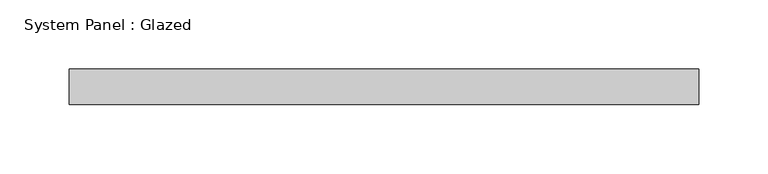
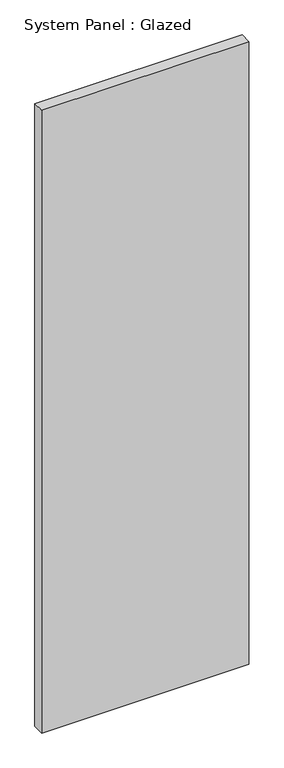
"""IFC4 building model written with IfcOpenShell, lengths in millimetres: plate geometry, System Panel : Glazed."""

from ifc_helpers import new_model, si_unit, origin, origin_with_axes, place, context, project, spatial, polyline, outline, extrude, source, transform, mapped, element, save


def system_panel_glazed_e446b74d(model_context):
    return source(origin(), model_context, "Body", "SweptSolid", [
        extrude(outline(polyline([(227.0125, 19.05), (-227.0125, 19.05), (-227.0125, 44.45), (227.0125, 44.45), (227.0125, 19.05)])), origin_with_axes(), (0.0, 0.0, 1.0), 1442.0265415),
    ])


if __name__ == "__main__":
    model = new_model("IFC4")
    model_context = context("Model", 3, world=origin())
    ifc_project = project(units=[si_unit("LENGTHUNIT", "METRE", prefix="MILLI")], contexts=[model_context])
    site = spatial("IfcSite", under=ifc_project)
    building = spatial("IfcBuilding", under=site)
    placement = place(None, origin())
    system_panel_glazed_shape = system_panel_glazed_e446b74d(model_context)
    element("IfcPlate", 1, ObjectType="System Panel : Glazed", at=placement, inside=building, context=model_context, shape_type="MappedRepresentation", body=[
        mapped(system_panel_glazed_shape, transform((0.0, 0.0, 0.0), x_axis=(1.0, 0.0, 0.0), y_axis=(0.0, 1.0, 0.0), z_axis=(0.0, 0.0, 1.0))),
    ])
    save(model, "model.ifc")

# Revit data of these elements
# Type "System Panel : Glazed"
#   Construction Type Id = "GSP4R"
#   Analytic Construction = "1/8 in Pilkington single glazing"
#   Visual Light Transmittance = 0.9
#   Solar Heat Gain Coefficient = 0.86
#   Heat Transfer Coefficient (U) = 1.18115 BTU/(h·ft²·°F)
#   Define Thermal Properties by = 1
# Element 1 (IfcPlate, "System Panel : Glazed")
#   Materials on its faces: "Glass"
# Materials
#   "Glass": class "Glass", colour RGB 0 128 192, transparency 0.75, Description = "Soda Lime Glass", Cost = 0
